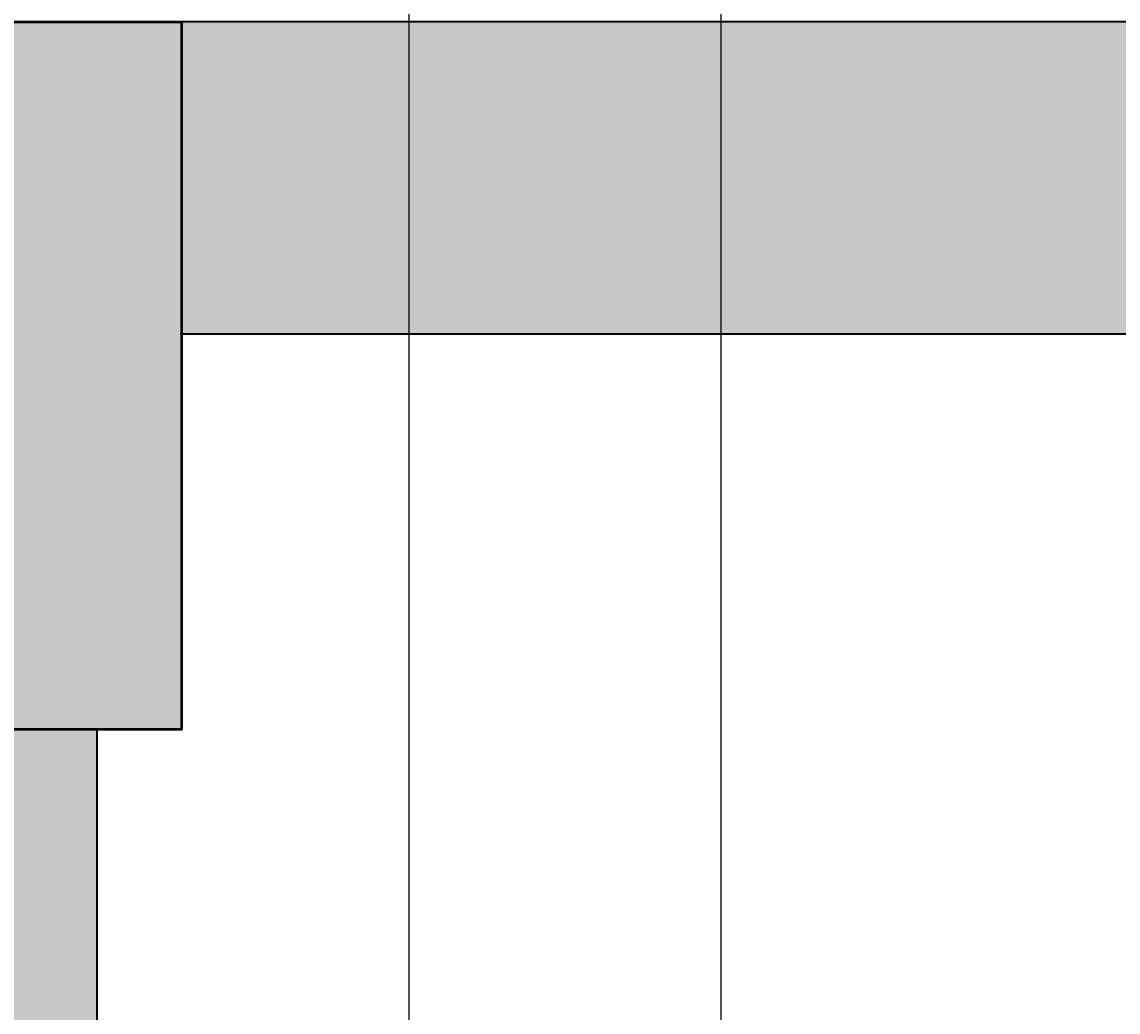
# Model space of a CAD drawing. Units: inches. Extents: x 1998 to 2588, y 1139 to 1977.
# Tile 72 of 134: x 2095 to 2126, y 1860 to 1889. Entities that reach past the tile are written whole.
import ezdxf

# ---------------------------------------------------------------- set-up
doc = ezdxf.new("R2010")
doc.units = ezdxf.units.IN
for name, color, linetype, lineweight in [('A-ANNO-DIMS', 2, 'Continuous', 18), ('A-COLS-PATT', 250, 'Continuous', 13), ('A-WALL-PATT', 252, 'Continuous', 13), ('COLUMN', 10, 'Continuous', 50), ('WALL', 200, 'Continuous', 35)]:
    doc.layers.add(name, color=color, linetype=linetype, lineweight=lineweight)
doc.styles.get("Standard").update_dxf_attribs({"font": 'arial.ttf'})
doc.dimstyles.get("Standard").update_dxf_attribs({"dimtxt": 0.18, "dimasz": 0.18, "dimexe": 0.18, "dimexo": 0.0625, "dimgap": 0.09, "dimtad": 0, "dimtih": 1, "dimtoh": 1, "dimdec": 4, "dimzin": 0, "dimdsep": 46, "dimtxsty": 'Standard', "dimcen": 0.09, "dimadec": 0, "dimazin": 0, "dimtfac": 1, "dimtdec": 4, "dimtofl": 0, "dimtmove": 0, "dimatfit": 3, "dimfxl": 1, "dimtolj": 1, "dimtzin": 0, "dimarcsym": 0})

# ---------------------------------------------------------------- blocks, each defined once
blk = doc.blocks.new('*D40')
at = {"layer": 'A-ANNO-DIMS', "color": 0, "lineweight": -2, "transparency": 16777216}
for p, q in [((2105.973, 1628.541), (2105.973, 1977.362)), ((2114.973, 1628.804), (2114.973, 1977.362)), ((2106.153, 1977.182), (2110.324, 1977.182)), ((2114.793, 1977.182), (2110.622, 1977.182))]:
    blk.add_line(p, q, dxfattribs=at)
at = {"layer": 'A-ANNO-DIMS', "color": 0, "transparency": 16777216}
for points in [[(2106.153, 1977.212), (2106.153, 1977.152), (2105.973, 1977.182)], [(2114.793, 1977.212), (2114.793, 1977.152), (2114.973, 1977.182)]]:
    blk.add_solid(points, dxfattribs=at)
at = {"layer": 'Defpoints', "color": 0, "transparency": 16777216}
for p in [(2114.973, 1977.182), (2114.973, 1628.742), (2105.973, 1628.478)]:
    blk.add_point(p, dxfattribs=at)
at = {"layer": 'A-ANNO-DIMS', "color": 0, "transparency": 16777216, "insert": (2110.473, 1977.182), "char_height": 0.18, "attachment_point": 5}
blk.add_mtext('\\A1;9', dxfattribs=at)

msp = doc.modelspace()

# ---------------------------------------------------------------- hatches: boundary and pattern name
at = {"layer": 'A-COLS-PATT'}
h = msp.add_hatch(color=256, dxfattribs=at)
h.dxf.hatch_style = 1
h.paths.add_polyline_path([(2099.4125, 1888.7324), (2087.9729, 1888.7324), (2087.9729, 1868.3278), (2099.4125, 1868.3278)])
h.paths.add_polyline_path([(2234.4125, 1888.7324), (2222.9729, 1888.7324), (2222.9729, 1868.3278), (2234.4125, 1868.3278)])
h.paths.add_polyline_path([(2341.4729, 1886.637), (2330.0332, 1886.637), (2330.0332, 1866.2324), (2341.4729, 1866.2324)])
h.paths.add_polyline_path([(2507.8006, 1882.7324), (2487.396, 1882.7324), (2487.396, 1871.2927), (2507.8006, 1871.2927)])
h.paths.add_polyline_path([(2510.9729, 1766.672), (2490.5682, 1766.672), (2490.5682, 1755.2324), (2510.9729, 1755.2324)])
h.paths.add_polyline_path([(2345.9729, 1759.7324), (2334.5332, 1759.7324), (2334.5332, 1739.3278), (2345.9729, 1739.3278)])
h.paths.add_polyline_path([(2234.4125, 1774.3318), (2222.9729, 1774.3318), (2222.9729, 1753.9272), (2234.4125, 1753.9272)])
h.paths.add_polyline_path([(2099.4125, 1775.637), (2087.9729, 1775.637), (2087.9729, 1755.2324), (2099.4125, 1755.2324)])
h.paths.add_polyline_path([(2098.0956, 1593.7241), (2077.691, 1593.7241), (2077.691, 1582.2845), (2098.0956, 1582.2845)])
h.paths.add_polyline_path([(2227.4729, 1604.637), (2216.0332, 1604.637), (2216.0332, 1584.2324), (2227.4729, 1584.2324)])
h.paths.add_polyline_path([(2345.9729, 1647.5211), (2334.5332, 1647.5211), (2334.5332, 1627.1165), (2345.9729, 1627.1165)])
h.paths.add_polyline_path([(2522.3775, 1641.2324), (2501.9729, 1641.2324), (2501.9729, 1629.7927), (2522.3775, 1629.7927)])
h.paths.add_polyline_path([(2522.3775, 1480.7324), (2501.9729, 1480.7324), (2501.9729, 1469.2927), (2522.3775, 1469.2927)])
h.paths.add_polyline_path([(2345.9729, 1488.5616), (2334.5332, 1488.5616), (2334.5332, 1468.1569), (2345.9729, 1468.1569)])
h.paths.add_polyline_path([(2234.4125, 1486.137), (2227.4729, 1486.137), (2227.4729, 1465.7324), (2234.4125, 1465.7324)])
h.paths.add_polyline_path([(2227.4729, 1486.137), (2222.9729, 1486.137), (2222.9729, 1465.7324), (2227.4729, 1465.7324)])
h.paths.add_polyline_path([(2108.3775, 1470.2324), (2087.9729, 1470.2324), (2087.9729, 1458.7927), (2108.3775, 1458.7927)])
h.paths.add_polyline_path([(2096.9729, 1365.5012), (2087.9729, 1365.5012), (2087.9729, 1345.0966), (2096.9729, 1345.0966)])
h.paths.add_polyline_path([(2087.9729, 1365.5012), (2085.5332, 1365.5012), (2085.5332, 1345.0966), (2087.9729, 1345.0966)])
h.paths.add_polyline_path([(2234.4125, 1285.137), (2222.9729, 1285.137), (2222.9729, 1264.7324), (2234.4125, 1264.7324)])
h.paths.add_polyline_path([(2345.9729, 1285.137), (2334.5332, 1285.137), (2334.5332, 1264.7324), (2345.9729, 1264.7324)])
h.paths.add_polyline_path([(2503.1458, 1240.172), (2482.7412, 1240.172), (2482.7412, 1228.7324), (2503.1458, 1228.7324)])
h.paths.add_polyline_path([(2510.9729, 1369.172), (2490.5682, 1369.172), (2490.5682, 1357.7324), (2510.9729, 1357.7324)])
at = {"layer": 'A-WALL-PATT'}
h = msp.add_hatch(color=256, dxfattribs=at)
h.dxf.hatch_style = 1
h.paths.add_polyline_path([(2222.9729, 1888.7324), (2099.4125, 1888.7324), (2099.4125, 1879.7324), (2222.9729, 1879.7324)])
h.paths.add_polyline_path([(2096.9729, 1868.3278), (2087.9729, 1868.3278), (2087.9729, 1775.637), (2096.9729, 1775.637)])
h.paths.add_polyline_path([(2227.4729, 1868.3278), (2222.9729, 1868.3278), (2222.9729, 1774.3318), (2227.4729, 1774.3318)])
h.paths.add_polyline_path([(2188.3019, 1759.7324), (2138.6074, 1759.7324), (2099.4125, 1759.7324), (2099.4125, 1755.2324), (2176.9729, 1755.2324), (2188.3019, 1755.2324)])
h.paths.add_polyline_path([(2087.9729, 1759.7324), (2059.4729, 1759.7324), (2059.4729, 1702.7324), (2087.9729, 1702.7324), (2087.9729, 1707.2324), (2063.9729, 1707.2324), (2063.9729, 1755.2324), (2087.9729, 1755.2324)])
h.paths.add_polyline_path([(2096.9729, 1755.2324), (2087.9729, 1755.2324), (2087.9729, 1707.2324), (2096.9729, 1707.2324)])
h.paths.add_polyline_path([(2187.0461, 1707.2324), (2105.9729, 1707.2324), (2096.9729, 1707.2324), (2087.9729, 1707.2324), (2087.9729, 1702.7324), (2105.9729, 1702.7324), (2114.9729, 1702.7324), (2187.0461, 1702.7324)])
h.paths.add_polyline_path([(2181.4729, 1719.2028), (2176.9729, 1719.2028), (2176.9729, 1707.2324), (2181.4729, 1707.2324)])
h.paths.add_polyline_path([(2216.0332, 1588.7324), (2114.9729, 1588.7324), (2105.9729, 1588.7324), (2105.9729, 1584.2324), (2216.0332, 1584.2324)])
h.paths.add_polyline_path([(2077.691, 1588.7324), (2061.4729, 1588.7324), (2061.4729, 1584.2324), (2077.691, 1584.2324)])
h.paths.add_polyline_path([(2105.9729, 1588.7324), (2098.0956, 1588.7324), (2098.0956, 1584.2324), (2105.9729, 1584.2324)])
h.paths.add_polyline_path([(2114.9729, 1596.2642), (2110.1012, 1596.2642), (2105.9729, 1596.2642), (2105.9729, 1588.7324), (2114.9729, 1588.7324)])
h.paths.add_polyline_path([(2114.9729, 1584.2324), (2105.9729, 1584.2324), (2105.9729, 1580.249), (2110.1012, 1580.249), (2114.9729, 1580.249)])
h.paths.add_polyline_path([(2114.9729, 1547.7716), (2110.1012, 1547.7716, -0.0318759), (2105.9729, 1548.035), (2105.9729, 1470.2324), (2108.3775, 1470.2324), (2108.3775, 1465.7324), (2186.2943, 1465.7324), (2186.2943, 1470.2324), (2114.9729, 1470.2324)])
h.paths.add_polyline_path([(2227.4729, 1584.2324), (2222.9729, 1584.2324), (2222.9729, 1486.137), (2227.4729, 1486.137)])
h.paths.add_polyline_path([(2295.4138, 1593.2324), (2227.4729, 1593.2324), (2227.4729, 1588.7324), (2295.4138, 1588.7324), (2295.4138, 1591.8729)])
h.paths.add_polyline_path([(2345.9729, 1627.1165), (2341.4729, 1627.1165), (2341.4729, 1593.2324), (2337.2869, 1593.2324), (2337.2869, 1591.8729), (2337.2869, 1588.7324), (2345.9729, 1588.7324)])
h.paths.add_polyline_path([(2291.9729, 1588.7324), (2287.4729, 1588.7324), (2287.4729, 1522.7324), (2291.9729, 1522.7324)])
h.paths.add_polyline_path([(2291.9729, 1522.7324), (2287.4729, 1522.7324), (2227.4729, 1522.7324), (2227.4729, 1518.2324), (2291.9729, 1518.2324)])
h.paths.add_polyline_path([(2295.7347, 1519.5919), (2295.7347, 1522.7324), (2291.9729, 1522.7324), (2291.9729, 1518.2324), (2295.7347, 1518.2324)])
h.paths.add_polyline_path([(2345.9729, 1522.7324), (2337.6078, 1522.7324), (2337.6078, 1519.5919), (2337.6078, 1518.2324), (2341.4729, 1518.2324), (2341.4729, 1488.5616), (2345.9729, 1488.5616)])
h.paths.add_polyline_path([(2345.9729, 1468.1569), (2341.4729, 1468.1569), (2341.4729, 1374.2324), (2227.4729, 1374.2324), (2227.4729, 1369.7324), (2345.9729, 1369.7324)])
h.paths.add_polyline_path([(2345.9729, 1369.7324), (2341.4729, 1369.7324), (2341.4729, 1362.2324), (2345.9729, 1362.2324)])
h.paths.add_polyline_path([(2345.9729, 1317.7324), (2345.9729, 1322.2324), (2341.4729, 1322.2324), (2341.4729, 1285.137), (2345.9729, 1285.137)], flags=17)
h.paths.add_polyline_path([(2356.2096, 1322.2324), (2345.9729, 1322.2324), (2345.9729, 1317.7324), (2356.2096, 1317.7324), (2356.2096, 1319.3088)], flags=17)
h.paths.add_polyline_path([(2393.9729, 1322.2324), (2375.6999, 1322.2324), (2375.6999, 1319.3088, -0.0202458), (2375.636, 1317.7324), (2393.9729, 1317.7324)], flags=17)
h.paths.add_polyline_path([(2398.4729, 1322.2324), (2393.9729, 1322.2324), (2393.9729, 1317.7324), (2393.9729, 1237.7324), (2345.9729, 1237.7324), (2345.9729, 1264.7324), (2341.4729, 1264.7324), (2341.4729, 1228.7324), (2393.9729, 1228.7324), (2482.7412, 1228.7324), (2482.7412, 1237.7324), (2398.4729, 1237.7324), (2398.4729, 1297.1029)])
h.paths.add_polyline_path([(2398.4729, 1362.2324), (2393.9729, 1362.2324), (2393.9729, 1357.7324), (2398.4729, 1357.7324)])
h.paths.add_polyline_path([(2345.9729, 1329.7549), (2341.4729, 1329.7549), (2341.4729, 1322.2324), (2345.9729, 1322.2324)])

# ---------------------------------------------------------------- linework, layer by layer
at = {"layer": 'COLUMN'}
msp.add_lwpolyline([(2087.9729, 1888.7324), (2099.4125, 1888.7324), (2099.4125, 1868.3278), (2087.9729, 1868.3278)], close=True, dxfattribs=at)
at = {"layer": 'WALL'}
for p, q in [((2227.4729, 1888.7324), (2087.9729, 1888.7324)), ((2222.9729, 1879.7324), (2099.4125, 1879.7324)), ((2096.9729, 1868.3278), (2096.9729, 1775.637))]:
    msp.add_line(p, q, dxfattribs=at)

# ---------------------------------------------------------------- dimensions: what is measured, and where the dimension line sits
at = {"layer": 'A-ANNO-DIMS'}
dim = msp.add_linear_dim(base=(2114.9729, 1977.1824), p1=(2105.9729, 1628.4781), p2=(2114.9729, 1628.7416), dimstyle='Standard', override={"dimdec": 0, "dimlfac": 1, "dimrnd": 0, "dimzin": 0, "dimdsep": 46, "dimlunit": 2}, dxfattribs=at)
dim.commit()
dim.dimension.update_dxf_attribs({"geometry": '*D40', "text_midpoint": (2110.4729, 1977.1824)})

doc.saveas('drawing.dxf')
